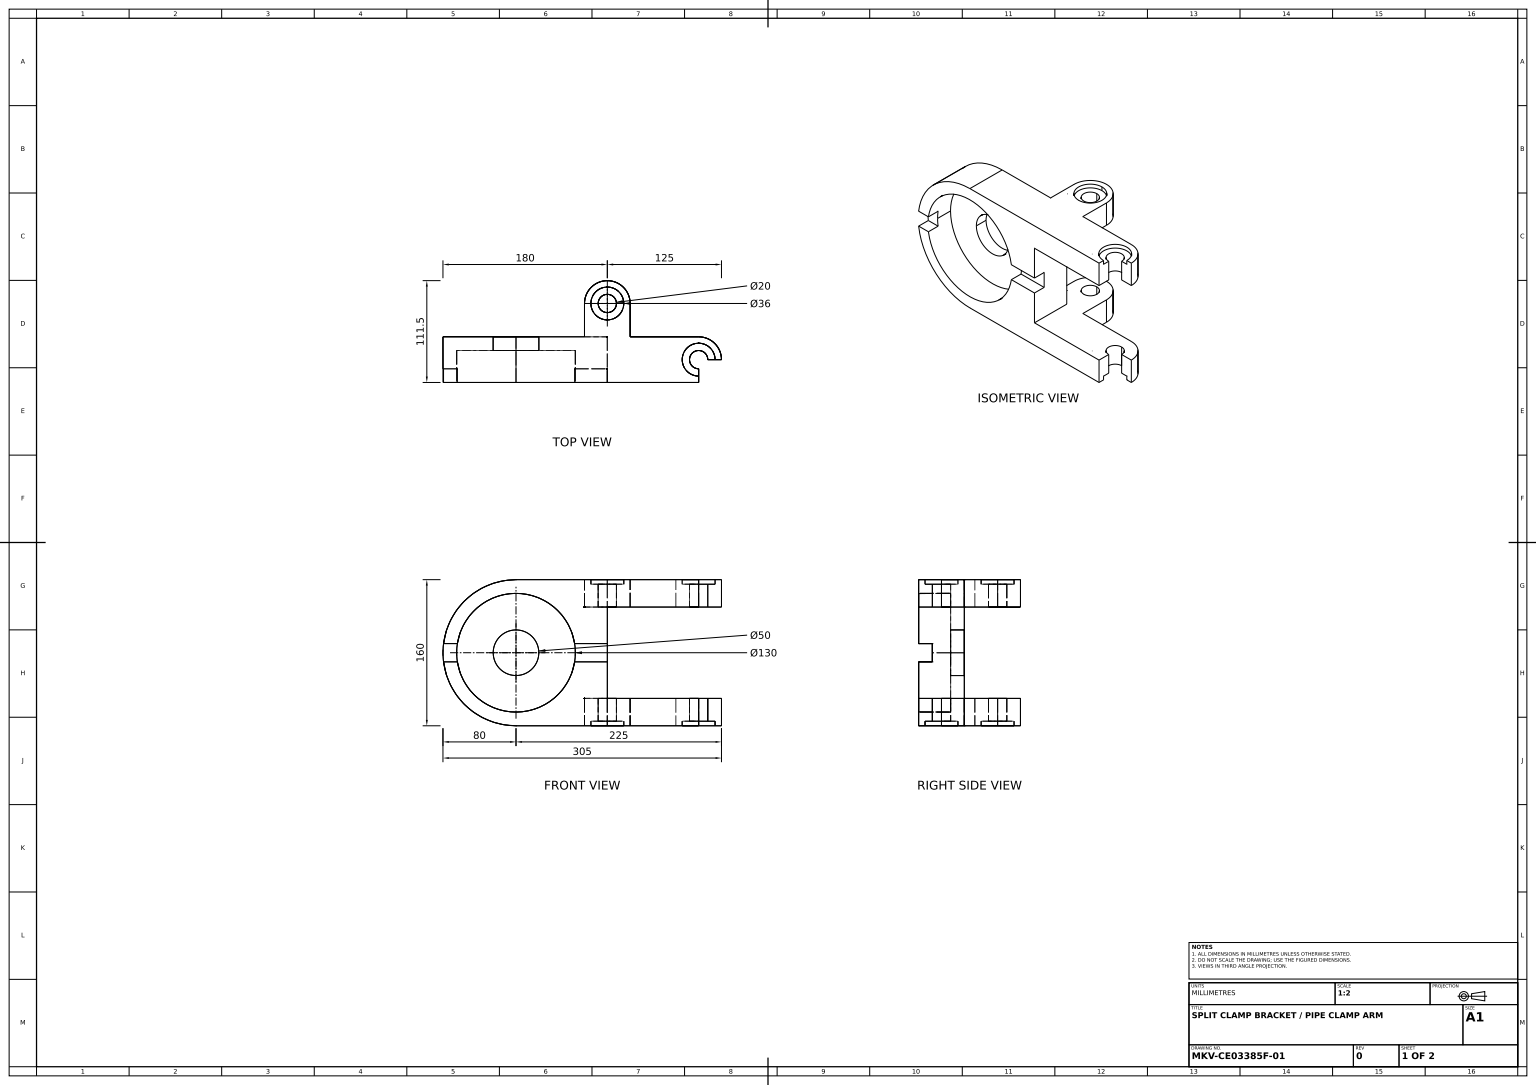
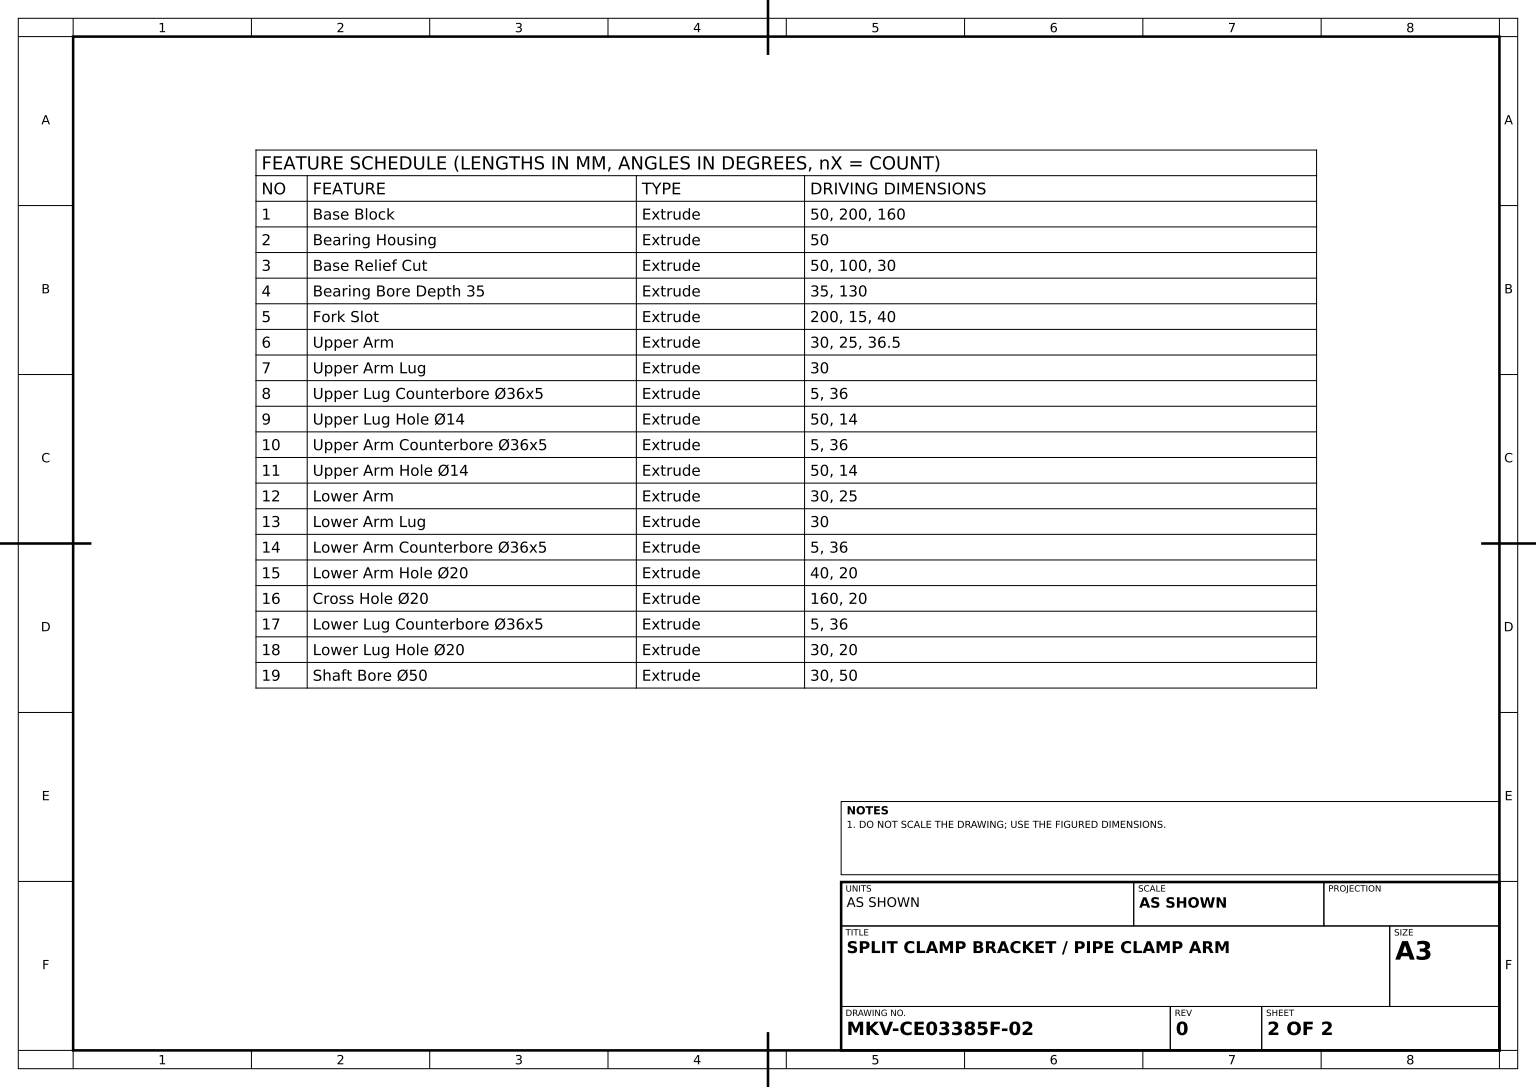
SolidWorks part; units mm, degrees
material "Plain Carbon Steel"
ref_plane "Front Plane" through (0, 0, 0) normal (0, 0, 1) x (1, 0, 0)
ref_plane "Top Plane" through (0, 0, 0) normal (0, 1, 0) x (1, 0, 0)
ref_plane "Right Plane" through (0, 0, 0) normal (1, 0, 0) x (0, 0, -1)
sketch "Base Block Sketch" plane through (0, 0, 0) normal (0, 0, 1) x (1, 0, 0)
  line L0 (0, 0) -> (200, 0)
  line L1 (200, 0) -> (200, 160)
  line L2 (200, 160) -> (0, 160)
  line L3 (0, 160) -> (0, 0)
  dimension "D1" = 200
  dimension "D2" = 160
extrude "Base Block" add sketch "Base Block Sketch" along normal blind 50
sketch "Bearing Housing Sketch" plane through (0, 0, 50) normal (0, 0, 1) x (1, 0, 0)
  line L0 (0, 160) -> (0, 0) construction
  line L1 (0, 160) -> (0, 0)
  arc A0 (0, 160) -> (0, 0) centre (0, 80) ccw
extrude "Bearing Housing" add sketch "Bearing Housing Sketch" against normal blind 50
sketch "Base Relief Cut Sketch" plane through (0, 0, 50) normal (0, 0, 1) x (1, 0, 0)
  line L0 (200, 160) -> (0, 160) construction
  line L1 (200, 0) -> (200, 160) construction
  line L2 (200, 130) -> (100, 130)
  line L3 (100, 130) -> (100, 30)
  line L4 (100, 30) -> (200, 30)
  line L5 (200, 30) -> (200, 130)
  dimension "D1" = 100
  dimension "D2" = 30
extrude "Base Relief Cut" cut sketch "Base Relief Cut Sketch" against normal blind 50
sketch "Bearing Bore Sketch" plane through (0, 0, 50) normal (0, 0, 1) x (1, 0, 0)
  circle A0 centre (0, 80) radius 65
  dimension "D1" = 130
extrude "Bearing Bore Depth 35" cut sketch "Bearing Bore Sketch" against normal blind 35
sketch "Fork Slot Sketch" plane through (100, 0, 0) normal (1, 0, 0) x (0, 0, -1)
  line L0 (-50, 80) -> (-50, 90)
  line L1 (-50, 130) -> (-50, 30) construction
  line L2 (-50, 90) -> (-35, 90)
  line L3 (-35, 90) -> (-35, 70)
  line L4 (-35, 70) -> (-50, 70)
  line L5 (-50, 70) -> (-50, 80)
  line L6 (0, 30) -> (-50, 30) construction
  dimension "D1" = 15
  dimension "D2" = 40
extrude "Fork Slot" cut sketch "Fork Slot Sketch" against normal blind 200
sketch "Upper Arm Sketch" plane through (0, 0, 0) normal (0, -1, 0) x (1, 0, 0)
  line L0 (125, 0) -> (100, 0)
  line L1 (0, 0) -> (200, 0) construction
  line L3 (75, -36.5) -> (75, 0)
  line L4 (125, -36.5) -> (125, 0)
  line L5 (75, 0) -> (100, 0)
  arc A0 (75, -36.5) -> (125, -36.5) centre (100, -36.5) ccw
  dimension "D1" = 50
  dimension "D2" = 25
  dimension "D3" = 36.5
extrude "Upper Arm" add sketch "Upper Arm Sketch" against normal blind 30
sketch "Upper Arm Lug Sketch" plane through (0, 160, 0) normal (0, 1, 0) x (1, 0, 0)
  line L2 (75, 36.5) -> (75, 0)
  line L3 (125, 36.5) -> (125, 0)
  line L4 (125, 0) -> (75, 0)
  arc A0 (125, 36.5) -> (75, 36.5) centre (100, 36.5) ccw
  dimension "D1" = 50
extrude "Upper Arm Lug" add sketch "Upper Arm Lug Sketch" against normal blind 30
sketch "Upper Lug Counterbore Sketch" plane through (0, 160, 0) normal (0, 1, 0) x (1, 0, 0)
  circle A0 centre (100, 36.5) radius 18
  dimension "D1" = 36
  dimension "D2" = 36
extrude "Upper Lug Counterbore Ø36x5" cut sketch "Upper Lug Counterbore Sketch" against normal blind 5
sketch "Upper Lug Hole Sketch" plane through (0, 155, 0) normal (0, 1, 0) x (1, 0, 0)
  circle A0 centre (100, 36.5) radius 7
  dimension "D1" = 14
  dimension "D2" = 14
extrude "Upper Lug Hole Ø14" cut sketch "Upper Lug Hole Sketch" against normal blind 50
sketch "Upper Arm Counterbore Sketch" plane through (0, 0, 0) normal (0, -1, 0) x (1, 0, 0)
  circle A0 centre (100, -36.5) radius 18
  dimension "D1" = 36
  dimension "D2" = 36
extrude "Upper Arm Counterbore Ø36x5" cut sketch "Upper Arm Counterbore Sketch" against normal blind 5
sketch "Upper Arm Hole Sketch" plane through (0, 5, 0) normal (0, -1, 0) x (1, 0, 0)
  circle A0 centre (100, -36.5) radius 7
  dimension "D1" = 14
  dimension "D2" = 14
extrude "Upper Arm Hole Ø14" cut sketch "Upper Arm Hole Sketch" against normal blind 50
sketch "Lower Arm Sketch" plane through (0, 0, 0) normal (0, -1, 0) x (1, 0, 0)
  line L0 (200, 50) -> (200, 0) construction
  line L1 (225, 25) -> (200, 25)
  line L2 (200, 25) -> (200, 50)
  arc A0 (200, 50) -> (225, 25) centre (200, 25) ccw
  dimension "D1" = 50
  dimension "D2" = 25
extrude "Lower Arm" add sketch "Lower Arm Sketch" against normal blind 30
sketch "Lower Arm Lug Sketch" plane through (0, 160, 0) normal (0, 1, 0) x (1, 0, 0)
  line L0 (200, -25) -> (225, -25)
  line L1 (200, -50) -> (200, 0) construction
  line L2 (200, -25) -> (200, 0)
  arc A0 (225, -25) -> (200, 0) centre (200, -25) ccw
  dimension "D1" = 50
extrude "Lower Arm Lug" add sketch "Lower Arm Lug Sketch" against normal blind 30
sketch "Lower Arm Counterbore Sketch" plane through (0, 0, 0) normal (0, -1, 0) x (1, 0, 0)
  circle A0 centre (200, 25) radius 18
  dimension "D1" = 36
  dimension "D2" = 36
extrude "Lower Arm Counterbore Ø36x5" cut sketch "Lower Arm Counterbore Sketch" against normal blind 5
sketch "Lower Arm Hole Sketch" plane through (0, 5, 0) normal (0, -1, 0) x (1, 0, 0)
  circle A1 centre (200, 25) radius 10
  dimension "D1" = 20
  dimension "D2" = 20
extrude "Lower Arm Hole Ø20" cut sketch "Lower Arm Hole Sketch" against normal blind 40
sketch "Cross Hole Sketch" plane through (0, 5, 0) normal (0, -1, 0) x (1, 0, 0)
  circle A0 centre (100, -36.5) radius 10
  dimension "D1" = 20
  dimension "D2" = 20
extrude "Cross Hole Ø20" cut sketch "Cross Hole Sketch" against normal blind 160
sketch "Lower Lug Counterbore Sketch" plane through (0, 160, 0) normal (0, 1, 0) x (1, 0, 0)
  circle A0 centre (200, -25) radius 18
  dimension "D1" = 36
  dimension "D2" = 36
extrude "Lower Lug Counterbore Ø36x5" cut sketch "Lower Lug Counterbore Sketch" against normal blind 5
sketch "Lower Lug Hole Sketch" plane through (0, 160, 0) normal (0, 1, 0) x (1, 0, 0)
  circle A0 centre (200, -25) radius 10
  dimension "D1" = 20
  dimension "D2" = 20
extrude "Lower Lug Hole Ø20" cut sketch "Lower Lug Hole Sketch" against normal blind 30
sketch "Shaft Bore Sketch" plane through (0, 0, 15) normal (0, 0, 1) x (1, 0, 0)
  circle A0 centre (0, 80) radius 25
  dimension "D1" = 50
  dimension "D2" = 50
extrude "Shaft Bore Ø50" cut sketch "Shaft Bore Sketch" against normal blind 30
